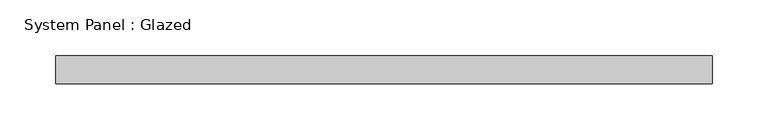
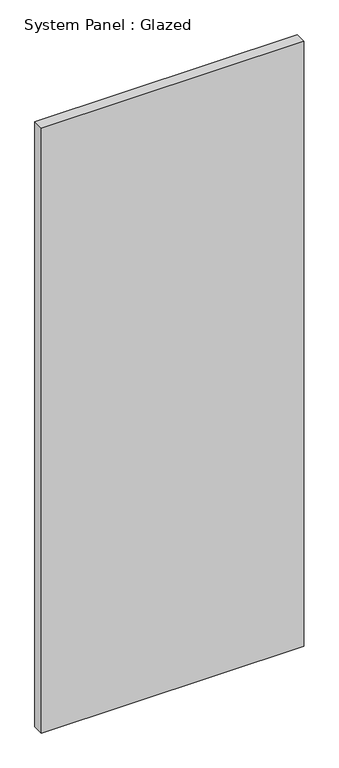
"""IFC4 building model written with IfcOpenShell, lengths in millimetres: plate geometry, System Panel : Glazed."""

from ifc_helpers import new_model, si_unit, origin, origin_with_axes, place, context, project, spatial, polyline, outline, extrude, source, transform, mapped, element, save


def system_panel_glazed_d0271aee(model_context):
    return source(origin(), model_context, "Body", "SweptSolid", [
        extrude(outline(polyline([(295.275, 19.05), (-295.275, 19.05), (-295.275, 44.45), (295.275, 44.45), (295.275, 19.05)])), origin_with_axes(), (0.0, 0.0, 1.0), 1439.7320436),
    ])


if __name__ == "__main__":
    model = new_model("IFC4")
    model_context = context("Model", 3, world=origin())
    ifc_project = project(units=[si_unit("LENGTHUNIT", "METRE", prefix="MILLI")], contexts=[model_context])
    site = spatial("IfcSite", under=ifc_project)
    building = spatial("IfcBuilding", under=site)
    placement = place(None, origin())
    system_panel_glazed_shape = system_panel_glazed_d0271aee(model_context)
    element("IfcPlate", 1, ObjectType="System Panel : Glazed", at=placement, inside=building, context=model_context, shape_type="MappedRepresentation", body=[
        mapped(system_panel_glazed_shape, transform((0.0, 0.0, 0.0), x_axis=(1.0, 0.0, 0.0), y_axis=(0.0, 1.0, 0.0), z_axis=(0.0, 0.0, 1.0))),
    ])
    save(model, "model.ifc")

# Revit data of these elements
# Type "System Panel : Glazed"
#   Construction Type Id = "GSP4R"
#   Analytic Construction = "1/8 in Pilkington single glazing"
#   Visual Light Transmittance = 0.9
#   Solar Heat Gain Coefficient = 0.86
#   Heat Transfer Coefficient (U) = 1.18115 BTU/(h·ft²·°F)
#   Define Thermal Properties by = 1
# Element 1 (IfcPlate, "System Panel : Glazed")
#   Materials on its faces: "Glass"
# Materials
#   "Glass": class "Glass", colour RGB 0 128 192, transparency 0.75, Description = "Soda Lime Glass", Cost = 0
